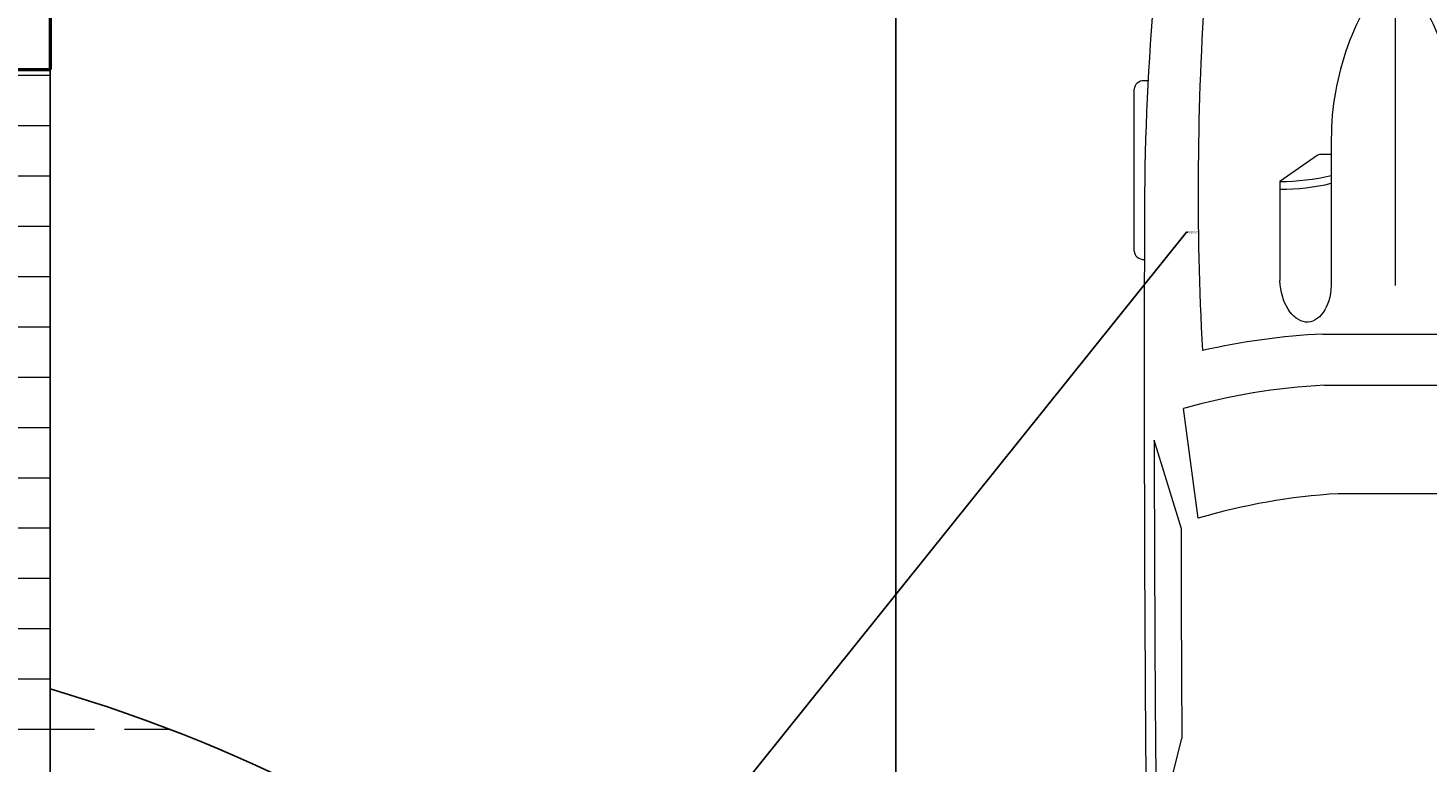
# Model space of a CAD drawing. Units: inches. Extents: x 5375 to 6084, y 16106 to 17259.
# Tile 7 of 32: x 5705 to 5844, y 16292 to 16365. Entities that reach past the tile are written whole.
import ezdxf

# ---------------------------------------------------------------- set-up
doc = ezdxf.new("R2010")
doc.units = ezdxf.units.IN
for name, color, linetype, lineweight in [('A-ANNO-DIMS', 2, 'Continuous', 18), ('C-PKNG-VEHI', 7, 'Continuous', 13), ('C-PVMT', 7, 'Continuous', 25), ('C-PVMT-PATT', 2, 'Continuous', 13), ('WALL', 6, 'Continuous', 50)]:
    doc.layers.add(name, color=color, linetype=linetype, lineweight=lineweight)
doc.styles.get("Standard").update_dxf_attribs({"font": 'arial.ttf'})
doc.dimstyles.get("Standard").update_dxf_attribs({"dimtxt": 0.18, "dimasz": 0.18, "dimexe": 0.18, "dimexo": 0.0625, "dimgap": 0.09, "dimtad": 0, "dimtih": 1, "dimtoh": 1, "dimdec": 4, "dimzin": 0, "dimdsep": 46, "dimtxsty": 'Standard', "dimcen": 0.09, "dimadec": 0, "dimazin": 0, "dimtfac": 1, "dimtdec": 4, "dimtofl": 0, "dimtmove": 0, "dimatfit": 3, "dimfxl": 1, "dimtolj": 1, "dimtzin": 0, "dimarcsym": 0})

# ---------------------------------------------------------------- blocks, each defined once
blk = doc.blocks.new('*U9')
for p, q in [((58.92, -10.77), (58.92, 10.77)), ((66.55, -10.53), (66.55, 10.53)), ((82.74, 8.5), (82.74, -8.5)), ((0, 0), (51.68, 0)), ((29.77, -9.51), (51.68, -9.51)), ((32.12, -9.51), (32.12, -11.15)), ((32.27, -11.63), (36.13, -17.17)), ((36.13, -17.17), (50.94, -17.17)), ((86.41, -29.35), (70.03, -31.54)), ((87.99, -31.87), (74.76, -35.92)), ((134.31, -35.6), (119.29, -31.78)), ((21.1, -37.41), (21.1, -36.83)), ((47.8, -37.39), (47.8, -37.41)), ((46.55, -38.89), (22.35, -38.89))]:
    blk.add_line(p, q)
for centre, major_axis, start_param, end_param in [((29.77, -46.66), (0, 56.17), 0, 0.590319), ((29.77, 46.66), (0, 56.17), 2.551274, 3.141593), ((13.04, -17.01), (0, -27.42), 1.564964, 1.848039), ((14.2, -17.01), (0, -27.42), 1.564964, 1.848039), ((149.6, -2.8), (0, -79.58), -1.499151, -1.230623), ((32.75, -11.15), (0, -0.74), 4.712389, 5.403472), ((134.4, -5.39), (0, -89.78), -1.510751, -1.307889), ((135.29, -5.39), (0, -81.77), -1.50788, -1.245306), ((37.47, 593.96), (0, -623.33), -0.059319, 0.045547), ((95.79, 3666.35), (0, -3698.24), -0.002505, 0.007544), ((41.19, 490.86), (0, -528.23), -0.075598, -0.00281), ((22.35, -37.41), (0, 1.48), 1.570796, 3.141593), ((64.48, 10555.62), (0, 10593.03), 3.138796, 3.15499), ((46.55, -37.41), (0, -1.48), 0, 1.570796), ((64.48, 10555.62), (0, -10591.55), 0.001152, 0.007828)]:
    blk.add_ellipse(centre, major_axis=major_axis, ratio=0.842304, start_param=start_param, end_param=end_param)
at = {"extrusion": (0, 0, -1)}
blk.add_ellipse((50.79, -13.34), major_axis=(6.34, 0.36), ratio=0.603834, start_param=-1.395552, end_param=1.581315, dxfattribs=at)
blk = doc.blocks.new('*D38')
at = {"layer": 'A-ANNO-DIMS', "color": 0, "lineweight": -2, "transparency": 16777216}
for p, q in [((5791.62, 16513.52), (5791.62, 16106.48)), ((5707.62, 16507.52), (5707.62, 16106.48)), ((5707.8, 16106.66), (5749.4, 16106.66)), ((5791.44, 16106.66), (5749.84, 16106.66))]:
    blk.add_line(p, q, dxfattribs=at)
at = {"layer": 'A-ANNO-DIMS', "color": 0, "transparency": 16777216}
for points in [[(5707.8, 16106.69), (5707.8, 16106.63), (5707.62, 16106.66)], [(5791.44, 16106.69), (5791.44, 16106.63), (5791.62, 16106.66)]]:
    blk.add_solid(points, dxfattribs=at)
at = {"layer": 'Defpoints', "color": 0, "transparency": 16777216}
for p in [(5791.62, 16513.58), (5707.62, 16507.58), (5791.62, 16106.66)]:
    blk.add_point(p, dxfattribs=at)
at = {"layer": 'A-ANNO-DIMS', "color": 0, "transparency": 16777216, "insert": (5749.62, 16106.66), "char_height": 0.18, "attachment_point": 5}
blk.add_mtext('\\A1;84', dxfattribs=at)
blk = doc.blocks.new('*D51')
at = {"layer": 'A-ANNO-DIMS', "color": 0, "lineweight": -2, "transparency": 16777216}
for p, q in [((5820.47, 16344.39), (5761.62, 16271.02)), ((5820.65, 16344.39), (5820.47, 16344.39)), ((5663.14, 16148.34), (5663.32, 16148.34)), ((5663.23, 16148.25), (5663.23, 16148.43))]:
    blk.add_line(p, q, dxfattribs=at)
at = {"layer": 'A-ANNO-DIMS', "color": 0, "transparency": 16777216}
blk.add_solid([(5761.59, 16271.03), (5761.64, 16271), (5761.5, 16270.88)], dxfattribs=at)
at = {"layer": 'Defpoints', "color": 0, "transparency": 16777216}
for p in [(5761.5, 16270.88), (5663.23, 16148.34)]:
    blk.add_point(p, dxfattribs=at)
at = {"layer": 'A-ANNO-DIMS', "color": 0, "transparency": 16777216, "insert": (5821.2, 16344.39), "char_height": 0.18, "attachment_point": 5}
blk.add_mtext('\\A1;R157.07', dxfattribs=at)

msp = doc.modelspace()

# ---------------------------------------------------------------- hatches: boundary and pattern name
at = {"layer": 'C-PVMT-PATT'}
h = msp.add_hatch(dxfattribs=at)
h.set_pattern_fill('AR-B816C', color=256)
h.paths.add_polyline_path([(5707.6199, 16360.5793), (5479.6199, 16360.5793), (5479.6199, 16221.3785), (5802.2897, 16221.3785, 0.20288708), (5707.6199, 16299.0135)])
h = msp.add_hatch(dxfattribs=at)
h.set_pattern_fill('ACAD_ISO08W100', color=256)
h.paths.add_polyline_path([(5707.6199, 16360.5793), (5479.6199, 16360.5793), (5479.6199, 16221.3785), (5802.2897, 16221.3785, 0.20288708), (5707.6199, 16299.0135)])

# ---------------------------------------------------------------- linework, layer by layer
at = {"layer": 'C-PVMT'}
msp.add_line((5707.6199, 16360.5793), (5707.6199, 16299.0135), dxfattribs=at)
msp.add_arc((5663.2298, 16148.3446), 157.072, 27.708351, 73.583948, dxfattribs=at)
at = {"layer": 'WALL'}
for p in [(5707.6199, 16402.5793), (5470.6199, 16360.5793)]:
    msp.add_line(p, (5707.6199, 16360.5793), dxfattribs=at)

# ---------------------------------------------------------------- block references
at = {"layer": 'C-PKNG-VEHI', "xscale": 0.6659567702331713, "yscale": 0.6659567702331713, "zscale": 0.6659567702331713, "rotation": 270}
msp.add_blockref('*U9', (5841.1969, 16373.5119), dxfattribs=at)

# ---------------------------------------------------------------- dimensions: what is measured, and where the dimension line sits
at = {"layer": 'A-ANNO-DIMS'}
dim = msp.add_linear_dim(base=(5791.6199, 16106.6631), p1=(5707.6199, 16507.5793), p2=(5791.6199, 16513.5793), dimstyle='Standard', override={"dimdec": 0, "dimlfac": 1, "dimrnd": 0, "dimzin": 0, "dimdsep": 46, "dimlunit": 2}, dxfattribs=at)
dim.commit()
dim.dimension.update_dxf_attribs({"geometry": '*D38', "text_midpoint": (5749.6199, 16106.6631)})
dim = msp.add_radius_dim(center=(5663.2298, 16148.3446), mpoint=(5761.504, 16270.8753), dimstyle='Standard', override={"dimdec": 2, "dimlfac": 1, "dimrnd": 0, "dimzin": 0, "dimdsep": 46, "dimlunit": 2}, dxfattribs=at)
dim.commit()
dim.dimension.update_dxf_attribs({"geometry": '*D51', "text_midpoint": (5821.1984, 16344.3937), "dimtype": 164})

doc.saveas('drawing.dxf')
